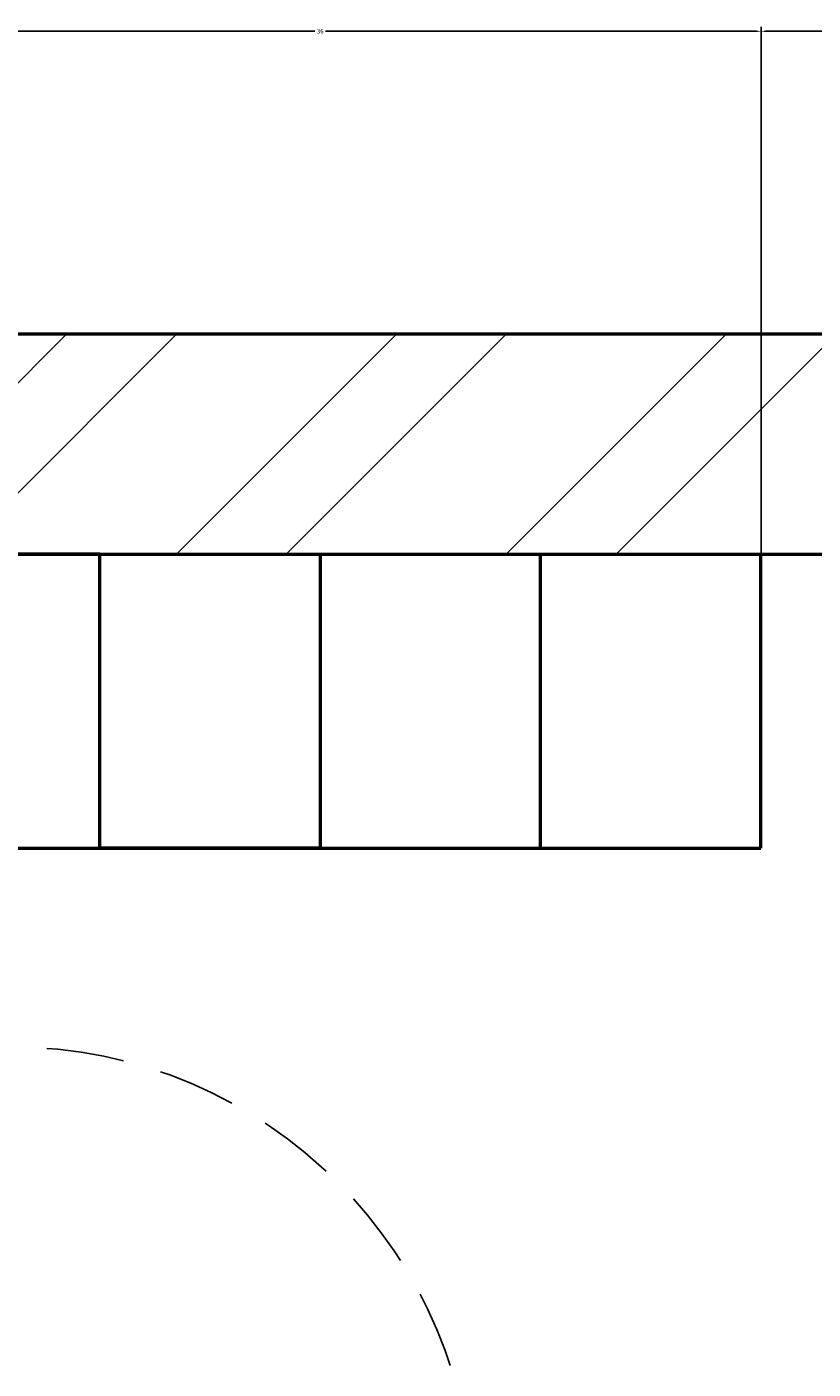
# Model space of a CAD drawing. Units: inches. Extents: x 2812 to 3051, y 1398 to 1659.
# Tile 56 of 65: x 2911 to 2944, y 1605 to 1659. Entities that reach past the tile are written whole.
import ezdxf

# ---------------------------------------------------------------- set-up
doc = ezdxf.new("R2010")
doc.units = ezdxf.units.IN
doc.linetypes.add('HIDDEN2', pattern=[4.7625, 3.175, -1.5875])
for name, color, linetype, lineweight in [('A-ANNO-DIMS', 2, 'Continuous', 18), ('S-CONC', 7, 'Continuous', 50), ('S-CONC-HIDN', 8, 'HIDDEN2', 25), ('S-CONC-PATT', 8, 'Continuous', 18)]:
    doc.layers.add(name, color=color, linetype=linetype, lineweight=lineweight)
doc.styles.get("Standard").update_dxf_attribs({"font": 'arial.ttf'})
doc.dimstyles.get("Standard").update_dxf_attribs({"dimtxt": 0.18, "dimasz": 0.18, "dimexe": 0.18, "dimexo": 0.0625, "dimgap": 0.09, "dimtad": 0, "dimtih": 1, "dimtoh": 1, "dimdec": 4, "dimzin": 0, "dimdsep": 46, "dimtxsty": 'Standard', "dimcen": 0.09, "dimadec": 0, "dimazin": 0, "dimtfac": 1, "dimtdec": 4, "dimtofl": 0, "dimtmove": 0, "dimatfit": 3, "dimfxl": 1, "dimtolj": 1, "dimtzin": 0, "dimarcsym": 0})

# ---------------------------------------------------------------- blocks, each defined once
blk = doc.blocks.new('*D19')
at = {"layer": 'A-ANNO-DIMS', "color": 0, "lineweight": -2, "transparency": 16777216}
for p, q in [((2905.385, 1625.882), (2905.385, 1659.35)), ((2941.385, 1625.882), (2941.385, 1659.35)), ((2905.565, 1659.17), (2923.166, 1659.17)), ((2941.205, 1659.17), (2923.604, 1659.17))]:
    blk.add_line(p, q, dxfattribs=at)
at = {"layer": 'A-ANNO-DIMS', "color": 0, "transparency": 16777216}
for points in [[(2905.565, 1659.2), (2905.565, 1659.14), (2905.385, 1659.17)], [(2941.205, 1659.2), (2941.205, 1659.14), (2941.385, 1659.17)]]:
    blk.add_solid(points, dxfattribs=at)
at = {"layer": 'Defpoints', "color": 0, "transparency": 16777216}
for p in [(2941.385, 1659.17), (2905.385, 1625.82), (2941.385, 1625.82)]:
    blk.add_point(p, dxfattribs=at)
at = {"layer": 'A-ANNO-DIMS', "color": 0, "transparency": 16777216, "insert": (2923.385, 1659.17), "char_height": 0.18, "attachment_point": 5}
blk.add_mtext('\\A1;36', dxfattribs=at)
blk = doc.blocks.new('*D20')
at = {"layer": 'A-ANNO-DIMS', "color": 0, "lineweight": -2, "transparency": 16777216}
for p, q in [((2941.385, 1625.882), (2941.385, 1659.35)), ((2952.385, 1637.882), (2952.385, 1659.35)), ((2941.565, 1659.17), (2946.692, 1659.17)), ((2952.205, 1659.17), (2947.078, 1659.17))]:
    blk.add_line(p, q, dxfattribs=at)
at = {"layer": 'A-ANNO-DIMS', "color": 0, "transparency": 16777216}
for points in [[(2941.565, 1659.2), (2941.565, 1659.14), (2941.385, 1659.17)], [(2952.205, 1659.2), (2952.205, 1659.14), (2952.385, 1659.17)]]:
    blk.add_solid(points, dxfattribs=at)
at = {"layer": 'Defpoints', "color": 0, "transparency": 16777216}
for p in [(2952.385, 1659.17), (2952.385, 1637.82), (2941.385, 1625.82)]:
    blk.add_point(p, dxfattribs=at)
at = {"layer": 'A-ANNO-DIMS', "color": 0, "transparency": 16777216, "insert": (2946.885, 1659.17), "char_height": 0.18, "attachment_point": 5}
blk.add_mtext('\\A1;11', dxfattribs=at)

msp = doc.modelspace()

# ---------------------------------------------------------------- hatches: boundary and pattern name
at = {"layer": 'S-CONC-PATT'}
h = msp.add_hatch(dxfattribs=at)
h.set_pattern_fill('ANSI32', color=256)
h.paths.add_polyline_path([(3027.3849, 1646.82), (2835.3849, 1646.82), (2835.3849, 1603.2296), (2844.3849, 1603.2296), (2844.3849, 1637.82), (3018.3849, 1637.82), (3018.3849, 1602.5441), (3027.3849, 1602.5441)])
h.paths.add_polyline_path([(2844.3849, 1594.2296), (2835.3849, 1594.2296), (2835.3849, 1550.82), (3027.3849, 1550.82), (3027.3849, 1593.5441), (3018.3849, 1593.5441), (3018.3849, 1559.82), (2844.3849, 1559.82)])
h.paths.add_polyline_path([(2844.3849, 1482.0354), (2835.3849, 1482.0354), (2835.3849, 1463.4959), (2844.3849, 1463.4959)])
h.paths.add_polyline_path([(2844.3849, 1461.4959), (2835.3849, 1461.4959), (2835.3849, 1416.0354), (2844.3849, 1416.0354)])
h.paths.add_polyline_path([(3027.3849, 1482.0354), (3018.3849, 1482.0354), (3018.3849, 1463.2854), (3027.3849, 1463.2854)])
h.paths.add_polyline_path([(3027.3849, 1461.2854), (3018.3849, 1461.2854), (3018.3849, 1416.0354), (3027.3849, 1416.0354)])
h.paths.add_polyline_path([(2961.3849, 1448.4738), (2952.3849, 1448.4738), (2952.3849, 1416.0354), (2961.3849, 1416.0354)])
h.paths.add_polyline_path([(2961.3849, 1462.3026), (2952.3849, 1462.3026), (2952.3849, 1450.4738), (2961.3849, 1450.4738)])
h.paths.add_polyline_path([(2961.3849, 1472.0354), (2952.3849, 1472.0354), (2952.3849, 1462.3026), (2961.3849, 1462.3026)])

# ---------------------------------------------------------------- linework, layer by layer
at = {"layer": 'S-CONC'}
for p, q in [((2835.3849, 1646.82), (3027.3849, 1646.82)), ((2844.3849, 1637.82), (3018.3849, 1637.82)), ((2914.3849, 1637.82), (2905.3849, 1637.82)), ((2914.3849, 1625.82), (2914.3849, 1637.82)), ((2923.3849, 1637.82), (2923.3849, 1625.82)), ((2932.3849, 1625.82), (2932.3849, 1637.82)), ((2941.3849, 1625.82), (2941.3849, 1637.82)), ((2896.3849, 1625.82), (2941.3849, 1625.82)), ((2923.3849, 1625.82), (2914.3849, 1625.82))]:
    msp.add_line(p, q, dxfattribs=at)
at = {"layer": 'S-CONC-HIDN'}
msp.add_circle((2910.7415, 1598.82), 18.8884, dxfattribs=at)

# ---------------------------------------------------------------- dimensions: what is measured, and where the dimension line sits
at = {"layer": 'A-ANNO-DIMS'}
for base, p1, p2, picture, middle in [((2941.3849, 1659.17), (2905.3849, 1625.82), (2941.3849, 1625.82), '*D19', (2923.3849, 1659.17)), ((2952.3849, 1659.17), (2941.3849, 1625.82), (2952.3849, 1637.82), '*D20', (2946.8849, 1659.17))]:
    dim = msp.add_linear_dim(base=base, p1=p1, p2=p2, dimstyle='Standard', override={"dimdec": 0, "dimlfac": 1, "dimrnd": 0, "dimzin": 0, "dimdsep": 46, "dimlunit": 2}, dxfattribs=at)
    dim.commit()
    dim.dimension.update_dxf_attribs({"geometry": picture, "text_midpoint": middle})

doc.saveas('drawing.dxf')
